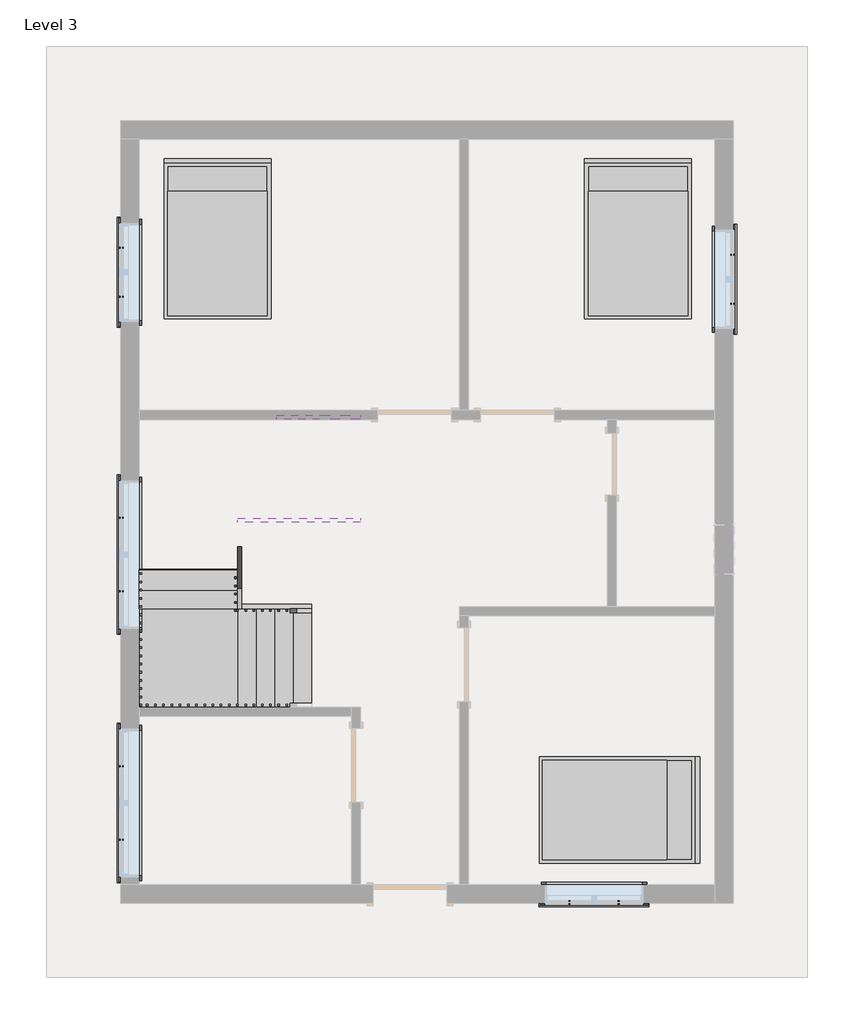
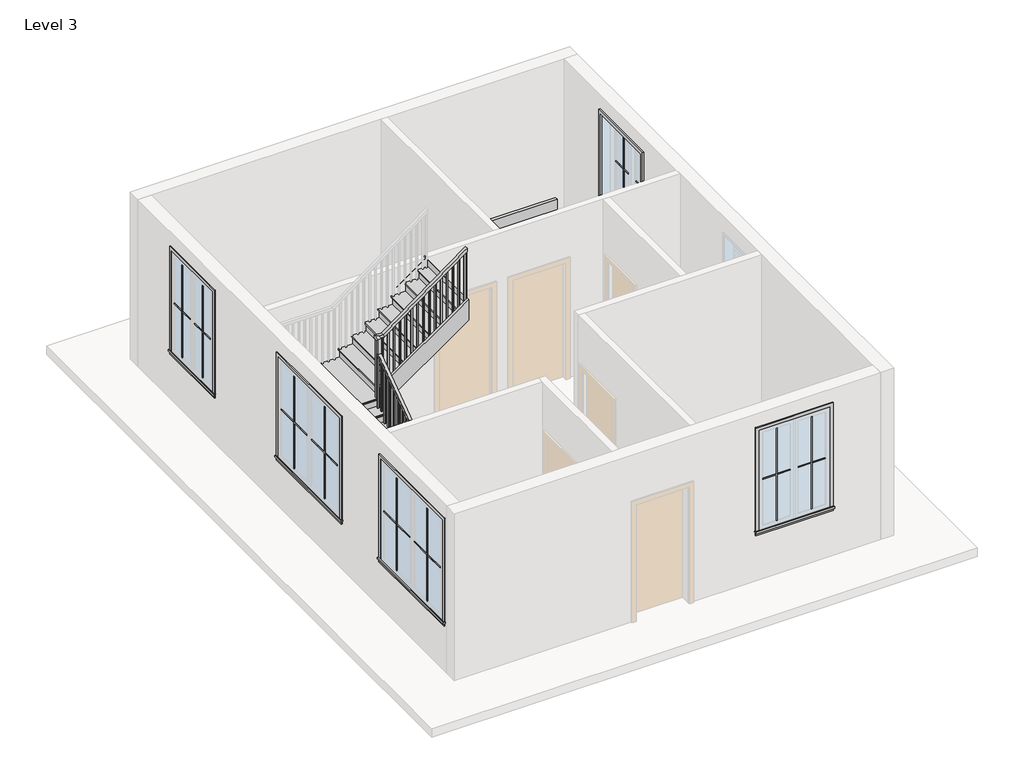
# One storey, part 3 of 3: 20 proxies, 5 members, 3 furniture elements, 1 railing, 1 stair flight.
"""IFC4 building model written with IfcOpenShell, lengths in millimetres."""

from ifc_helpers import new_model, si_unit, frame, origin, place, context, project, spatial, polyline, outline, extrude, faceted_brep, transform, mapped, element, save
from components import muntin_pattern_2x2_muntin_pattern_2x2_0a037076, muntin_pattern_2x2_muntin_pattern_2x2_e6f69628, muntin_pattern_2x2_muntin_pattern_2x2_2b4d9f72, muntin_pattern_2x2_muntin_pattern_2x2_ef995ed3, trim_window_exterior_flat_with_sill_b601e94a, trim_window_exterior_flat_with_sill_b7e4d11c, trim_window_interior_flat_picture_frame_bfefb25c, trim_window_interior_flat_picture_frame_936b8d2a, bed_17739_bed_17739_15c61121, stair_flight_424eac51

model = new_model("IFC4")

# Units and contexts
model_context = context("Model", 3, world=origin())
ifc_project = project(units=[si_unit("LENGTHUNIT", "METRE", prefix="MILLI")], contexts=[model_context])

# Site, building, storey
site = spatial("IfcSite", under=ifc_project)
building = spatial("IfcBuilding", under=site)
storey = spatial("IfcBuildingStorey", under=building, Name="Level 3", Elevation=6248.4)

# Proxies
placement = place(None, origin())
muntin_pattern_2x2_muntin_pattern_2x2_shape = muntin_pattern_2x2_muntin_pattern_2x2_0a037076(model_context)
element("IfcBuildingElementProxy", 1, Name="Muntin Pattern_2x2 : Muntin Pattern_2x2", ObjectType="Muntin Pattern_2x2 : Muntin Pattern_2x2", at=placement, inside=storey, context=model_context, shape_type="MappedRepresentation", body=[
    mapped(muntin_pattern_2x2_muntin_pattern_2x2_shape, transform((-5035.7855391, -4380.9248761, 7232.65), x_axis=(0.0, 1.0, 0.0), y_axis=(-1.0, 0.0, 0.0), z_axis=(0.0, 0.0, 1.0))),
])
element("IfcBuildingElementProxy", 2, Name="Muntin Pattern_2x2 : Muntin Pattern_2x2", ObjectType="Muntin Pattern_2x2 : Muntin Pattern_2x2", at=placement, inside=storey, context=model_context, shape_type="MappedRepresentation", body=[
    mapped(muntin_pattern_2x2_muntin_pattern_2x2_shape, transform((-5035.7855391, -1310.6998761, 7232.65), x_axis=(0.0, 1.0, 0.0), y_axis=(-1.0, 0.0, 0.0), z_axis=(0.0, 0.0, 1.0))),
])
muntin_pattern_2x2_muntin_pattern_2x2_2_shape = muntin_pattern_2x2_muntin_pattern_2x2_e6f69628(model_context)
element("IfcBuildingElementProxy", 3, Name="Muntin Pattern_2x2 : Muntin Pattern_2x2", ObjectType="Muntin Pattern_2x2 : Muntin Pattern_2x2", at=placement, inside=storey, context=model_context, shape_type="MappedRepresentation", body=[
    mapped(muntin_pattern_2x2_muntin_pattern_2x2_2_shape, transform((-5035.7855391, -3469.6998761, 7232.65), x_axis=(0.0, -1.0, 0.0), y_axis=(1.0, 0.0, 0.0), z_axis=(0.0, 0.0, 1.0))),
])
element("IfcBuildingElementProxy", 4, Name="Muntin Pattern_2x2 : Muntin Pattern_2x2", ObjectType="Muntin Pattern_2x2 : Muntin Pattern_2x2", at=placement, inside=storey, context=model_context, shape_type="MappedRepresentation", body=[
    mapped(muntin_pattern_2x2_muntin_pattern_2x2_2_shape, transform((-5035.7855391, -399.4748761, 7232.65), x_axis=(0.0, -1.0, 0.0), y_axis=(1.0, 0.0, 0.0), z_axis=(0.0, 0.0, 1.0))),
])
muntin_pattern_2x2_muntin_pattern_2x2_3_shape = muntin_pattern_2x2_muntin_pattern_2x2_2b4d9f72(model_context)
element("IfcBuildingElementProxy", 5, Name="Muntin Pattern_2x2 : Muntin Pattern_2x2", ObjectType="Muntin Pattern_2x2 : Muntin Pattern_2x2", at=placement, inside=storey, context=model_context, shape_type="MappedRepresentation", body=[
    mapped(muntin_pattern_2x2_muntin_pattern_2x2_3_shape, transform((1115.7769609, -5157.2123761, 7232.65), x_axis=(-1.0, 0.0, 0.0), y_axis=(0.0, -1.0, 0.0), z_axis=(0.0, 0.0, 1.0))),
])
element("IfcBuildingElementProxy", 6, Name="Muntin Pattern_2x2 : Muntin Pattern_2x2", ObjectType="Muntin Pattern_2x2 : Muntin Pattern_2x2", at=placement, inside=storey, context=model_context, shape_type="MappedRepresentation", body=[
    mapped(muntin_pattern_2x2_muntin_pattern_2x2_3_shape, transform((2527.0644609, 2851.7251239, 7232.65), x_axis=(0.0, -1.0, 0.0), y_axis=(1.0, 0.0, 0.0), z_axis=(0.0, 0.0, 1.0))),
])
element("IfcBuildingElementProxy", 7, Name="Muntin Pattern_2x2 : Muntin Pattern_2x2", ObjectType="Muntin Pattern_2x2 : Muntin Pattern_2x2", at=placement, inside=storey, context=model_context, shape_type="MappedRepresentation", body=[
    mapped(muntin_pattern_2x2_muntin_pattern_2x2_3_shape, transform((-5035.7855391, 2331.0251239, 7232.65), x_axis=(0.0, 1.0, 0.0), y_axis=(-1.0, 0.0, 0.0), z_axis=(0.0, 0.0, 1.0))),
])
muntin_pattern_2x2_muntin_pattern_2x2_4_shape = muntin_pattern_2x2_muntin_pattern_2x2_ef995ed3(model_context)
element("IfcBuildingElementProxy", 8, Name="Muntin Pattern_2x2 : Muntin Pattern_2x2", ObjectType="Muntin Pattern_2x2 : Muntin Pattern_2x2", at=placement, inside=storey, context=model_context, shape_type="MappedRepresentation", body=[
    mapped(muntin_pattern_2x2_muntin_pattern_2x2_4_shape, transform((509.3519609, -5157.2123761, 7232.65), x_axis=(1.0, 0.0, 0.0), y_axis=(0.0, 1.0, 0.0), z_axis=(0.0, 0.0, 1.0))),
])
element("IfcBuildingElementProxy", 9, Name="Muntin Pattern_2x2 : Muntin Pattern_2x2", ObjectType="Muntin Pattern_2x2 : Muntin Pattern_2x2", at=placement, inside=storey, context=model_context, shape_type="MappedRepresentation", body=[
    mapped(muntin_pattern_2x2_muntin_pattern_2x2_4_shape, transform((2527.0644609, 2245.3001239, 7232.65), x_axis=(0.0, 1.0, 0.0), y_axis=(-1.0, 0.0, 0.0), z_axis=(0.0, 0.0, 1.0))),
])
element("IfcBuildingElementProxy", 10, Name="Muntin Pattern_2x2 : Muntin Pattern_2x2", ObjectType="Muntin Pattern_2x2 : Muntin Pattern_2x2", at=placement, inside=storey, context=model_context, shape_type="MappedRepresentation", body=[
    mapped(muntin_pattern_2x2_muntin_pattern_2x2_4_shape, transform((-5035.7855391, 2937.4501239, 7232.65), x_axis=(0.0, -1.0, 0.0), y_axis=(1.0, 0.0, 0.0), z_axis=(0.0, 0.0, 1.0))),
])
trim_window_exterior_flat_with_sill_shape = trim_window_exterior_flat_with_sill_b601e94a(model_context)
element("IfcBuildingElementProxy", 11, Name="Trim-Window-Exterior-Flat : with Sill", ObjectType="Trim-Window-Exterior-Flat : with Sill", at=placement, inside=storey, context=model_context, shape_type="MappedRepresentation", body=[
    mapped(trim_window_exterior_flat_with_sill_shape, transform((-5045.3105391, -3925.3123761, 8991.6), x_axis=(0.0, -1.0, 0.0), y_axis=(0.0, 0.0, 1.0), z_axis=(-1.0, 0.0, 0.0))),
])
element("IfcBuildingElementProxy", 12, Name="Trim-Window-Exterior-Flat : with Sill", ObjectType="Trim-Window-Exterior-Flat : with Sill", at=placement, inside=storey, context=model_context, shape_type="MappedRepresentation", body=[
    mapped(trim_window_exterior_flat_with_sill_shape, transform((-5045.3105391, -855.0873761, 8991.6), x_axis=(0.0, -1.0, 0.0), y_axis=(0.0, 0.0, 1.0), z_axis=(-1.0, 0.0, 0.0))),
])
trim_window_exterior_flat_with_sill_2_shape = trim_window_exterior_flat_with_sill_b7e4d11c(model_context)
element("IfcBuildingElementProxy", 13, Name="Trim-Window-Exterior-Flat : with Sill", ObjectType="Trim-Window-Exterior-Flat : with Sill", at=placement, inside=storey, context=model_context, shape_type="MappedRepresentation", body=[
    mapped(trim_window_exterior_flat_with_sill_2_shape, transform((812.5644609, -5166.7373761, 8991.6), x_axis=(1.0, 0.0, 0.0), y_axis=(0.0, 0.0, 1.0), z_axis=(0.0, -1.0, 0.0))),
])
element("IfcBuildingElementProxy", 14, Name="Trim-Window-Exterior-Flat : with Sill", ObjectType="Trim-Window-Exterior-Flat : with Sill", at=placement, inside=storey, context=model_context, shape_type="MappedRepresentation", body=[
    mapped(trim_window_exterior_flat_with_sill_2_shape, transform((2536.5894609, 2548.5126239, 8991.6), x_axis=(0.0, 1.0, 0.0), y_axis=(0.0, 0.0, 1.0), z_axis=(1.0, 0.0, 0.0))),
])
element("IfcBuildingElementProxy", 15, Name="Trim-Window-Exterior-Flat : with Sill", ObjectType="Trim-Window-Exterior-Flat : with Sill", at=placement, inside=storey, context=model_context, shape_type="MappedRepresentation", body=[
    mapped(trim_window_exterior_flat_with_sill_2_shape, transform((-5045.3105391, 2634.2376239, 8991.6), x_axis=(0.0, -1.0, 0.0), y_axis=(0.0, 0.0, 1.0), z_axis=(-1.0, 0.0, 0.0))),
])
trim_window_interior_flat_picture_frame_shape = trim_window_interior_flat_picture_frame_bfefb25c(model_context)
element("IfcBuildingElementProxy", 16, Name="Trim-Window-Interior-Flat : Picture Frame", ObjectType="Trim-Window-Interior-Flat : Picture Frame", at=placement, inside=storey, context=model_context, shape_type="MappedRepresentation", body=[
    mapped(trim_window_interior_flat_picture_frame_shape, transform((-4816.7105391, -3925.3123761, 8991.6), x_axis=(0.0, 1.0, 0.0), y_axis=(0.0, 0.0, 1.0), z_axis=(1.0, 0.0, 0.0))),
])
element("IfcBuildingElementProxy", 17, Name="Trim-Window-Interior-Flat : Picture Frame", ObjectType="Trim-Window-Interior-Flat : Picture Frame", at=placement, inside=storey, context=model_context, shape_type="MappedRepresentation", body=[
    mapped(trim_window_interior_flat_picture_frame_shape, transform((-4816.7105391, -855.0873761, 8991.6), x_axis=(0.0, 1.0, 0.0), y_axis=(0.0, 0.0, 1.0), z_axis=(1.0, 0.0, 0.0))),
])
trim_window_interior_flat_picture_frame_2_shape = trim_window_interior_flat_picture_frame_936b8d2a(model_context)
element("IfcBuildingElementProxy", 18, Name="Trim-Window-Interior-Flat : Picture Frame", ObjectType="Trim-Window-Interior-Flat : Picture Frame", at=placement, inside=storey, context=model_context, shape_type="MappedRepresentation", body=[
    mapped(trim_window_interior_flat_picture_frame_2_shape, transform((812.5644609, -4938.1373761, 8991.6), x_axis=(-1.0, 0.0, 0.0), y_axis=(0.0, 0.0, 1.0), z_axis=(0.0, 1.0, 0.0))),
])
element("IfcBuildingElementProxy", 19, Name="Trim-Window-Interior-Flat : Picture Frame", ObjectType="Trim-Window-Interior-Flat : Picture Frame", at=placement, inside=storey, context=model_context, shape_type="MappedRepresentation", body=[
    mapped(trim_window_interior_flat_picture_frame_2_shape, transform((2307.9894609, 2548.5126239, 8991.6), x_axis=(0.0, -1.0, 0.0), y_axis=(0.0, 0.0, 1.0), z_axis=(-1.0, 0.0, 0.0))),
])
element("IfcBuildingElementProxy", 20, Name="Trim-Window-Interior-Flat : Picture Frame", ObjectType="Trim-Window-Interior-Flat : Picture Frame", at=placement, inside=storey, context=model_context, shape_type="MappedRepresentation", body=[
    mapped(trim_window_interior_flat_picture_frame_2_shape, transform((-4816.7105391, 2634.2376239, 8991.6), x_axis=(0.0, 1.0, 0.0), y_axis=(0.0, 0.0, 1.0), z_axis=(1.0, 0.0, 0.0))),
])

# Furniture
bed_17739_bed_17739_shape = bed_17739_bed_17739_15c61121(model_context)
element("IfcFurniture", 21, ObjectType="Bed_17739 : Bed_17739", at=placement, inside=storey, context=model_context, shape_type="MappedRepresentation", body=[
    mapped(bed_17739_bed_17739_shape, transform((-3845.1605391, 3024.7626239, 6248.4), x_axis=(1.0, 0.0, 0.0), y_axis=(0.0, 1.0, 0.0), z_axis=(0.0, 0.0, 1.0))),
])
element("IfcFurniture", 22, ObjectType="Bed_17739 : Bed_17739", at=placement, inside=storey, context=model_context, shape_type="MappedRepresentation", body=[
    mapped(bed_17739_bed_17739_shape, transform((1355.4894609, 3024.7626239, 6248.4), x_axis=(1.0, 0.0, 0.0), y_axis=(0.0, 1.0, 0.0), z_axis=(0.0, 0.0, 1.0))),
])
element("IfcFurniture", 23, ObjectType="Bed_17739 : Bed_17739", at=placement, inside=storey, context=model_context, shape_type="MappedRepresentation", body=[
    mapped(bed_17739_bed_17739_shape, transform((1101.4894609, -4011.0373761, 6248.4), x_axis=(0.0, -1.0, 0.0), y_axis=(1.0, 0.0, 0.0), z_axis=(0.0, 0.0, 1.0))),
])

# Members
element("IfcMember", 24, ObjectType="Stringer - 2\" Width", at=placement, inside=storey, context=model_context, shape_type="SweptSolid", body=[
    extrude(outline(polyline([(6248.4, -2683.1105391), (6398.9087903, -2683.1105391), (6398.9087903, -3112.2707489), (6248.4, -2897.7957228), (6248.4, -2683.1105391)])), frame((0.0, -2791.8373761, 0.0), z_axis=(0.0, 1.0, 0.0), x_axis=(0.0, 0.0, 1.0)), (0.0, 0.0, 1.0), 50.8),
])
element("IfcMember", 25, ObjectType="Stringer - 2\" Width", at=placement, inside=storey, context=model_context, shape_type="SweptSolid", body=[
    extrude(outline(polyline([(8575.8856495, -2580.7583047), (8931.8489938, -2073.5105391), (9304.2117181, -2073.5105391), (8575.8856495, -3111.3751869), (8575.8856495, -2580.7583047)])), frame((0.0, 814.9626239, 0.0), z_axis=(0.0, 1.0, 0.0), x_axis=(0.0, 0.0, 1.0)), (0.0, 0.0, 1.0), 50.8),
])
element("IfcMember", 26, ObjectType="Stringer - 2\" Width", at=placement, inside=storey, context=model_context, shape_type="SweptSolid", body=[
    extrude(outline(polyline([(6248.4, -2683.1105391), (6470.106455, -2683.1105391), (7076.1415427, -3546.7105391), (6703.7788184, -3546.7105391), (6248.4, -2897.7957228), (6248.4, -2683.1105391)])), frame((0.0, -1521.8373761, 0.0), z_axis=(0.0, 1.0, 0.0), x_axis=(0.0, 0.0, 1.0)), (0.0, 0.0, 1.0), 50.8),
])
element("IfcMember", 27, ObjectType="Stringer - 2\" Width", at=placement, inside=storey, context=model_context, shape_type="SweptSolid", body=[
    extrude(outline(polyline([(-1521.8373761, 6898.7564629), (-1521.8373761, 7273.9327137), (-455.0373761, 8039.5786467), (-455.0373761, 7664.4023959), (-1521.8373761, 6898.7564629)])), frame((-3597.5105391, 0.0, 0.0), z_axis=(1.0, 0.0, 0.0), x_axis=(0.0, 1.0, 0.0)), (0.0, 0.0, 1.0), 50.8),
])
element("IfcMember", 28, ObjectType="Stringer - 2\" Width", at=placement, inside=storey, context=model_context, shape_type="SweptSolid", body=[
    extrude(outline(polyline([(8234.7380339, -3597.5105391), (7862.3753096, -3597.5105391), (8931.8489938, -2073.5105391), (9304.2117181, -2073.5105391), (8234.7380339, -3597.5105391)])), frame((0.0, -455.0373761, 0.0), z_axis=(0.0, 1.0, 0.0), x_axis=(0.0, 0.0, 1.0)), (0.0, 0.0, 1.0), 50.8),
])

# Railing
element("IfcRailing", 29, ObjectType="Handrail - Rectangular", at=placement, inside=storey, context=model_context, shape_type="SolidModel", body=[
    faceted_brep([(-2683.1105391, -1572.6373761, 7323.2210526), (-2683.1105391, -1572.6373761, 7261.1605986), (-2683.1105391, -1521.8373761, 7261.1605986), (-2683.1105391, -1521.8373761, 7323.2210526), (-3521.3105391, -1572.6373761, 7911.4315789), (-3572.1105391, -1572.6373761, 7885.0202477), (-3572.1105391, -1521.8373761, 7885.0202477), (-3521.3105391, -1521.8373761, 7911.4315789), (-3521.3105391, -1572.6373761, 8180.015311), (-3572.1105391, -1572.6373761, 8129.215311), (-3572.1105391, -1521.8373761, 8129.215311), (-3521.3105391, -1521.8373761, 8180.015311), (-3648.3105391, -1572.6373761, 8180.015311), (-3648.3105391, -1572.6373761, 8129.215311), (-3597.5105391, -1521.8373761, 8129.215311), (-3597.5105391, -1521.8373761, 8180.015311), (-3648.3105391, -1445.6373761, 8180.015311), (-3648.3105391, -1429.2944467, 8129.215311), (-3597.5105391, -1429.2944467, 8129.215311), (-3597.5105391, -1445.6373761, 8180.015311), (-3648.3105391, -480.4373761, 8872.7425837), (-3648.3105391, -429.6373761, 8846.6725387), (-3597.5105391, -429.6373761, 8846.6725387), (-3597.5105391, -480.4373761, 8872.7425837), (-3648.3105391, -480.4373761, 9144.0), (-3648.3105391, -429.6373761, 9093.2), (-3597.5105391, -429.6373761, 9093.2), (-3597.5105391, -480.4373761, 9144.0), (-3648.3105391, -353.4373761, 9144.0), (-3648.3105391, -353.4373761, 9093.2), (-3597.5105391, -404.2373761, 9093.2), (-3597.5105391, -404.2373761, 9144.0), (-3521.3105391, -353.4373761, 9144.0), (-3504.6160355, -353.4373761, 9093.2), (-3504.6160355, -404.2373761, 9093.2), (-3521.3105391, -404.2373761, 9144.0), (-2073.5105391, -353.4373761, 10210.8), (-2073.5105391, -404.2373761, 10210.8), (-2073.5105391, -404.2373761, 10147.6987868), (-2073.5105391, -353.4373761, 10147.6987868)], [[[0, 1, 2, 3]], [[1, 0, 4, 5]], [[2, 1, 5, 6]], [[3, 2, 6, 7]], [[0, 3, 7, 4]], [[5, 4, 8, 9]], [[6, 5, 9, 10]], [[7, 6, 10, 11]], [[4, 7, 11, 8]], [[9, 8, 12, 13]], [[10, 9, 13, 14]], [[11, 10, 14, 15]], [[8, 11, 15, 12]], [[13, 12, 16, 17]], [[14, 13, 17, 18]], [[15, 14, 18, 19]], [[12, 15, 19, 16]], [[17, 16, 20, 21]], [[18, 17, 21, 22]], [[19, 18, 22, 23]], [[16, 19, 23, 20]], [[21, 20, 24, 25]], [[22, 21, 25, 26]], [[23, 22, 26, 27]], [[20, 23, 27, 24]], [[25, 24, 28, 29]], [[26, 25, 29, 30]], [[27, 26, 30, 31]], [[24, 27, 31, 28]], [[29, 28, 32, 33]], [[30, 29, 33, 34]], [[31, 30, 34, 35]], [[28, 31, 35, 32]], [[36, 37, 38, 39]], [[33, 32, 36, 39]], [[34, 33, 39, 38]], [[35, 34, 38, 37]], [[32, 35, 37, 36]]]),
    extrude(outline(polyline([(10136.0014184, -2089.3855391), (10121.9645763, -2108.4355391), (9135.9789474, -2108.4355391), (9135.9789474, -2089.3855391), (10136.0014184, -2089.3855391)])), frame((0.0, -388.3623761, 0.0), z_axis=(0.0, 1.0, 0.0), x_axis=(0.0, 0.0, 1.0)), (0.0, 0.0, 1.0), 19.05),
    extrude(outline(polyline([(10061.1382605, -2190.9855391), (10047.1014184, -2210.0355391), (9135.9789474, -2210.0355391), (9135.9789474, -2190.9855391), (10061.1382605, -2190.9855391)])), frame((0.0, -388.3623761, 0.0), z_axis=(0.0, 1.0, 0.0), x_axis=(0.0, 0.0, 1.0)), (0.0, 0.0, 1.0), 19.05),
    extrude(outline(polyline([(9986.2751026, -2292.5855391), (9972.2382605, -2311.6355391), (8975.5578947, -2311.6355391), (8975.5578947, -2292.5855391), (9986.2751026, -2292.5855391)])), frame((0.0, -388.3623761, 0.0), z_axis=(0.0, 1.0, 0.0), x_axis=(0.0, 0.0, 1.0)), (0.0, 0.0, 1.0), 19.05),
    extrude(outline(polyline([(9911.4119447, -2394.1855391), (9897.3751026, -2413.2355391), (8975.5578947, -2413.2355391), (8975.5578947, -2394.1855391), (9911.4119447, -2394.1855391)])), frame((0.0, -388.3623761, 0.0), z_axis=(0.0, 1.0, 0.0), x_axis=(0.0, 0.0, 1.0)), (0.0, 0.0, 1.0), 19.05),
    extrude(outline(polyline([(9836.5487868, -2495.7855391), (9822.5119447, -2514.8355391), (8815.1368421, -2514.8355391), (8815.1368421, -2495.7855391), (9836.5487868, -2495.7855391)])), frame((0.0, -388.3623761, 0.0), z_axis=(0.0, 1.0, 0.0), x_axis=(0.0, 0.0, 1.0)), (0.0, 0.0, 1.0), 19.05),
    extrude(outline(polyline([(9761.6856289, -2597.3855391), (9747.6487868, -2616.4355391), (8815.1368421, -2616.4355391), (8815.1368421, -2597.3855391), (9761.6856289, -2597.3855391)])), frame((0.0, -388.3623761, 0.0), z_axis=(0.0, 1.0, 0.0), x_axis=(0.0, 0.0, 1.0)), (0.0, 0.0, 1.0), 19.05),
    extrude(outline(polyline([(9686.822471, -2698.9855391), (9672.7856289, -2718.0355391), (8654.7157895, -2718.0355391), (8654.7157895, -2698.9855391), (9686.822471, -2698.9855391)])), frame((0.0, -388.3623761, 0.0), z_axis=(0.0, 1.0, 0.0), x_axis=(0.0, 0.0, 1.0)), (0.0, 0.0, 1.0), 19.05),
    extrude(outline(polyline([(9611.9593132, -2800.5855391), (9597.922471, -2819.6355391), (8654.7157895, -2819.6355391), (8654.7157895, -2800.5855391), (9611.9593132, -2800.5855391)])), frame((0.0, -388.3623761, 0.0), z_axis=(0.0, 1.0, 0.0), x_axis=(0.0, 0.0, 1.0)), (0.0, 0.0, 1.0), 19.05),
    extrude(outline(polyline([(9537.0961553, -2902.1855391), (9523.0593132, -2921.2355391), (8654.7157895, -2921.2355391), (8654.7157895, -2902.1855391), (9537.0961553, -2902.1855391)])), frame((0.0, -388.3623761, 0.0), z_axis=(0.0, 1.0, 0.0), x_axis=(0.0, 0.0, 1.0)), (0.0, 0.0, 1.0), 19.05),
    extrude(outline(polyline([(9462.2329974, -3003.7855391), (9448.1961553, -3022.8355391), (8494.2947368, -3022.8355391), (8494.2947368, -3003.7855391), (9462.2329974, -3003.7855391)])), frame((0.0, -388.3623761, 0.0), z_axis=(0.0, 1.0, 0.0), x_axis=(0.0, 0.0, 1.0)), (0.0, 0.0, 1.0), 19.05),
    extrude(outline(polyline([(9387.3698395, -3105.3855391), (9373.3329974, -3124.4355391), (8494.2947368, -3124.4355391), (8494.2947368, -3105.3855391), (9387.3698395, -3105.3855391)])), frame((0.0, -388.3623761, 0.0), z_axis=(0.0, 1.0, 0.0), x_axis=(0.0, 0.0, 1.0)), (0.0, 0.0, 1.0), 19.05),
    extrude(outline(polyline([(9312.5066816, -3206.9855391), (9298.4698395, -3226.0355391), (8333.8736842, -3226.0355391), (8333.8736842, -3206.9855391), (9312.5066816, -3206.9855391)])), frame((0.0, -388.3623761, 0.0), z_axis=(0.0, 1.0, 0.0), x_axis=(0.0, 0.0, 1.0)), (0.0, 0.0, 1.0), 19.05),
    extrude(outline(polyline([(9237.6435237, -3308.5855391), (9223.6066816, -3327.6355391), (8333.8736842, -3327.6355391), (8333.8736842, -3308.5855391), (9237.6435237, -3308.5855391)])), frame((0.0, -388.3623761, 0.0), z_axis=(0.0, 1.0, 0.0), x_axis=(0.0, 0.0, 1.0)), (0.0, 0.0, 1.0), 19.05),
    extrude(outline(polyline([(9162.7803658, -3410.1855391), (9148.7435237, -3429.2355391), (8173.4526316, -3429.2355391), (8173.4526316, -3410.1855391), (9162.7803658, -3410.1855391)])), frame((0.0, -388.3623761, 0.0), z_axis=(0.0, 1.0, 0.0), x_axis=(0.0, 0.0, 1.0)), (0.0, 0.0, 1.0), 19.05),
    extrude(outline(polyline([(9087.9172079, -3511.7855391), (9073.8803658, -3530.8355391), (8173.4526316, -3530.8355391), (8173.4526316, -3511.7855391), (9087.9172079, -3511.7855391)])), frame((0.0, -388.3623761, 0.0), z_axis=(0.0, 1.0, 0.0), x_axis=(0.0, 0.0, 1.0)), (0.0, 0.0, 1.0), 19.05),
    extrude(outline(polyline([(-3613.3855391, -439.1623761), (-3632.4355391, -439.1623761), (-3632.4355391, -420.1123761), (-3613.3855391, -420.1123761), (-3613.3855391, -439.1623761)])), frame((0.0, 0.0, 7852.6105263), z_axis=(0.0, 0.0, 1.0), x_axis=(1.0, 0.0, 0.0)), (0.0, 0.0, 1.0), 1240.5894737),
    extrude(outline(polyline([(-540.7623761, 8766.9177541), (-521.7123761, 8780.5900029), (-521.7123761, 7852.6105263), (-540.7623761, 7852.6105263), (-540.7623761, 8766.9177541)])), frame((-3632.4355391, 0.0, 0.0), z_axis=(1.0, 0.0, 0.0), x_axis=(0.0, 1.0, 0.0)), (0.0, 0.0, 1.0), 19.05),
    extrude(outline(polyline([(-642.3623761, 8693.9990938), (-623.3123761, 8707.6713426), (-623.3123761, 7692.1894737), (-642.3623761, 7692.1894737), (-642.3623761, 8693.9990938)])), frame((-3632.4355391, 0.0, 0.0), z_axis=(1.0, 0.0, 0.0), x_axis=(0.0, 1.0, 0.0)), (0.0, 0.0, 1.0), 19.05),
    extrude(outline(polyline([(-743.9623761, 8621.0804335), (-724.9123761, 8634.7526823), (-724.9123761, 7692.1894737), (-743.9623761, 7692.1894737), (-743.9623761, 8621.0804335)])), frame((-3632.4355391, 0.0, 0.0), z_axis=(1.0, 0.0, 0.0), x_axis=(0.0, 1.0, 0.0)), (0.0, 0.0, 1.0), 19.05),
    extrude(outline(polyline([(-845.5623761, 8548.1617732), (-826.5123761, 8561.834022), (-826.5123761, 7692.1894737), (-845.5623761, 7692.1894737), (-845.5623761, 8548.1617732)])), frame((-3632.4355391, 0.0, 0.0), z_axis=(1.0, 0.0, 0.0), x_axis=(0.0, 1.0, 0.0)), (0.0, 0.0, 1.0), 19.05),
    extrude(outline(polyline([(-947.1623761, 8475.2431129), (-928.1123761, 8488.9153617), (-928.1123761, 7531.7684211), (-947.1623761, 7531.7684211), (-947.1623761, 8475.2431129)])), frame((-3632.4355391, 0.0, 0.0), z_axis=(1.0, 0.0, 0.0), x_axis=(0.0, 1.0, 0.0)), (0.0, 0.0, 1.0), 19.05),
    extrude(outline(polyline([(-1048.7623761, 8402.3244526), (-1029.7123761, 8415.9967014), (-1029.7123761, 7531.7684211), (-1048.7623761, 7531.7684211), (-1048.7623761, 8402.3244526)])), frame((-3632.4355391, 0.0, 0.0), z_axis=(1.0, 0.0, 0.0), x_axis=(0.0, 1.0, 0.0)), (0.0, 0.0, 1.0), 19.05),
    extrude(outline(polyline([(-1150.3623761, 8329.4057923), (-1131.3123761, 8343.0780411), (-1131.3123761, 7371.3473684), (-1150.3623761, 7371.3473684), (-1150.3623761, 8329.4057923)])), frame((-3632.4355391, 0.0, 0.0), z_axis=(1.0, 0.0, 0.0), x_axis=(0.0, 1.0, 0.0)), (0.0, 0.0, 1.0), 19.05),
    extrude(outline(polyline([(-1251.9623761, 8256.487132), (-1232.9123761, 8270.1593808), (-1232.9123761, 7371.3473684), (-1251.9623761, 7371.3473684), (-1251.9623761, 8256.487132)])), frame((-3632.4355391, 0.0, 0.0), z_axis=(1.0, 0.0, 0.0), x_axis=(0.0, 1.0, 0.0)), (0.0, 0.0, 1.0), 19.05),
    extrude(outline(polyline([(-1353.5623761, 8183.5684718), (-1334.5123761, 8197.2407206), (-1334.5123761, 7210.9263158), (-1353.5623761, 7210.9263158), (-1353.5623761, 8183.5684718)])), frame((-3632.4355391, 0.0, 0.0), z_axis=(1.0, 0.0, 0.0), x_axis=(0.0, 1.0, 0.0)), (0.0, 0.0, 1.0), 19.05),
    extrude(outline(polyline([(-1455.1623761, 8110.6498115), (-1436.1123761, 8124.3220603), (-1436.1123761, 7210.9263158), (-1455.1623761, 7210.9263158), (-1455.1623761, 8110.6498115)])), frame((-3632.4355391, 0.0, 0.0), z_axis=(1.0, 0.0, 0.0), x_axis=(0.0, 1.0, 0.0)), (0.0, 0.0, 1.0), 19.05),
    extrude(outline(polyline([(-3587.9855391, -1537.7123761), (-3587.9855391, -1556.7623761), (-3607.0355391, -1556.7623761), (-3607.0355391, -1537.7123761), (-3587.9855391, -1537.7123761)])), frame((0.0, 0.0, 7050.5052632), z_axis=(0.0, 0.0, 1.0), x_axis=(1.0, 0.0, 0.0)), (0.0, 0.0, 1.0), 1078.7100478),
    extrude(outline(polyline([(7824.862353, -3486.3855391), (7838.230774, -3505.4355391), (6890.0842105, -3505.4355391), (6890.0842105, -3486.3855391), (7824.862353, -3486.3855391)])), frame((0.0, -1556.7623761, 0.0), z_axis=(0.0, 1.0, 0.0), x_axis=(0.0, 0.0, 1.0)), (0.0, 0.0, 1.0), 19.05),
    extrude(outline(polyline([(7753.5641074, -3384.7855391), (7766.9325284, -3403.8355391), (6890.0842105, -3403.8355391), (6890.0842105, -3384.7855391), (7753.5641074, -3384.7855391)])), frame((0.0, -1556.7623761, 0.0), z_axis=(0.0, 1.0, 0.0), x_axis=(0.0, 0.0, 1.0)), (0.0, 0.0, 1.0), 19.05),
    extrude(outline(polyline([(7682.2658617, -3283.1855391), (7695.6342828, -3302.2355391), (6729.6631579, -3302.2355391), (6729.6631579, -3283.1855391), (7682.2658617, -3283.1855391)])), frame((0.0, -1556.7623761, 0.0), z_axis=(0.0, 1.0, 0.0), x_axis=(0.0, 0.0, 1.0)), (0.0, 0.0, 1.0), 19.05),
    extrude(outline(polyline([(7610.9676161, -3181.5855391), (7624.3360372, -3200.6355391), (6729.6631579, -3200.6355391), (6729.6631579, -3181.5855391), (7610.9676161, -3181.5855391)])), frame((0.0, -1556.7623761, 0.0), z_axis=(0.0, 1.0, 0.0), x_axis=(0.0, 0.0, 1.0)), (0.0, 0.0, 1.0), 19.05),
    extrude(outline(polyline([(7539.6693705, -3079.9855391), (7553.0377916, -3099.0355391), (6569.2421053, -3099.0355391), (6569.2421053, -3079.9855391), (7539.6693705, -3079.9855391)])), frame((0.0, -1556.7623761, 0.0), z_axis=(0.0, 1.0, 0.0), x_axis=(0.0, 0.0, 1.0)), (0.0, 0.0, 1.0), 19.05),
    extrude(outline(polyline([(7468.3711249, -2978.3855391), (7481.7395459, -2997.4355391), (6569.2421053, -2997.4355391), (6569.2421053, -2978.3855391), (7468.3711249, -2978.3855391)])), frame((0.0, -1556.7623761, 0.0), z_axis=(0.0, 1.0, 0.0), x_axis=(0.0, 0.0, 1.0)), (0.0, 0.0, 1.0), 19.05),
    extrude(outline(polyline([(7397.0728793, -2876.7855391), (7410.4413003, -2895.8355391), (6408.8210526, -2895.8355391), (6408.8210526, -2876.7855391), (7397.0728793, -2876.7855391)])), frame((0.0, -1556.7623761, 0.0), z_axis=(0.0, 1.0, 0.0), x_axis=(0.0, 0.0, 1.0)), (0.0, 0.0, 1.0), 19.05),
    extrude(outline(polyline([(7325.7746337, -2775.1855391), (7339.1430547, -2794.2355391), (6408.8210526, -2794.2355391), (6408.8210526, -2775.1855391), (7325.7746337, -2775.1855391)])), frame((0.0, -1556.7623761, 0.0), z_axis=(0.0, 1.0, 0.0), x_axis=(0.0, 0.0, 1.0)), (0.0, 0.0, 1.0), 19.05),
    extrude(outline(polyline([(-3613.3855391, -388.3623761), (-3632.4355391, -388.3623761), (-3632.4355391, -369.3123761), (-3613.3855391, -369.3123761), (-3613.3855391, -388.3623761)])), frame((0.0, 0.0, 8013.0315789), z_axis=(0.0, 0.0, 1.0), x_axis=(1.0, 0.0, 0.0)), (0.0, 0.0, 1.0), 1080.1684211),
    extrude(outline(polyline([(-3613.3855391, -1537.7123761), (-3613.3855391, -1556.7623761), (-3632.4355391, -1556.7623761), (-3632.4355391, -1537.7123761), (-3613.3855391, -1537.7123761)])), frame((0.0, 0.0, 7050.5052632), z_axis=(0.0, 0.0, 1.0), x_axis=(1.0, 0.0, 0.0)), (0.0, 0.0, 1.0), 1078.7100478),
    extrude(outline(polyline([(10147.6987868, -2073.5105391), (10133.6619447, -2092.5605391), (9135.9789474, -2092.5605391), (9135.9789474, -2073.5105391), (10147.6987868, -2073.5105391)])), frame((0.0, -388.3623761, 0.0), z_axis=(0.0, 1.0, 0.0), x_axis=(0.0, 0.0, 1.0)), (0.0, 0.0, 1.0), 19.05),
    extrude(outline(polyline([(7261.1605986, -2683.1105391), (7274.5290196, -2702.1605391), (6408.8210526, -2702.1605391), (6408.8210526, -2683.1105391), (7261.1605986, -2683.1105391)])), frame((0.0, -1556.7623761, 0.0), z_axis=(0.0, 1.0, 0.0), x_axis=(0.0, 0.0, 1.0)), (0.0, 0.0, 1.0), 19.05),
])

# Stair flight
stair_flight_shape = stair_flight_424eac51(model_context)
element("IfcStairFlight", 30, ObjectType="2\" Tread 1\" Nosing 1/4\" Riser", at=placement, inside=storey, context=model_context, shape_type="MappedRepresentation", body=[
    mapped(stair_flight_shape, transform((0.0, 0.0, 0.0), x_axis=(1.0, 0.0, 0.0), y_axis=(0.0, 1.0, 0.0), z_axis=(0.0, 0.0, 1.0))),
])

save(model, "model.ifc")

# Revit data of these elements
# Type "Muntin Pattern_2x2 : Muntin Pattern_2x2"
#   Width [instance default] = 4' - 0"
#   Thickness = 0' - 0 1/2"
#   Height [instance default] = 4' - 0"
#   Distance = 0' - 0 3/4"
#   Interior Material [instance default] = none
#   Exterior Material [instance default] = none
#   Default Elevation = 0
# Type "Trim-Window-Exterior-Flat : with Sill"
#   Trim Width = 0' - 2 1/4"
#   Trim Thickness_Picture Frame = 0' - 1 1/4"
#   Trim Thickness_with Sill = 0' - 0 3/4"
#   Sill Thickness = 0' - 1 1/4"
#   Opening Width [instance default] = 2' - 0"
#   Opening Height [instance default] = 3' - 0"
#   Default Elevation = 4' - 0"
#   Sill = yes
#   Picture Frame = no
#   Trim Material [instance default] = none
# Type "Trim-Window-Interior-Flat : Picture Frame"
#   Trim Thickness_Picture Frame = 0' - 1 1/4"
#   Trim Width = 0' - 2 1/4"
#   Trim Thickness_with Sill = 0' - 0 3/4"
#   Sill Thickness = 0' - 1 1/4"
#   Opening Width [instance default] = 2' - 0"
#   Opening Height [instance default] = 3' - 0"
#   Default Elevation = 4' - 0"
#   Sill = no
#   Picture Frame = yes
#   Trim Material [instance default] = none
# Type "Bed_17739 : Bed_17739"
#   Default Elevation = 0
# Type "Handrail - Rectangular"
#   Assembly Code = "C2010400"
#   built-in parameter 1008612 = 0.0416667 (stored number, unit not read)
#   built-in parameter 1008611 = 0.0416667 (stored number, unit not read)
#   built-in parameter 1008609 = 0.333333 (stored number, unit not read)
#   built-in parameter 1008604 = 0.166667 (stored number, unit not read)
#   built-in parameter 1008603 = 0.166667 (stored number, unit not read)
#   Railing Height = 3' - 0"
#   built-in parameter 1008630 = 2
#   built-in parameter 1008610 = 2
#   built-in parameter 1008618 = Baluster - Square : 3/4"
# Elements 1, 2, 3, 4 (IfcBuildingElementProxy, "Muntin Pattern_2x2 : Muntin Pattern_2x2")
#   Width = 2' - 6 5/8"
#   Height = 5' - 6 1/2"
#   Interior Material = Wood - Stained
#   Exterior Material = Clad - White
#   Phase Created = New Construction
#   Materials on its faces: "Clad - White", "Wood - Stained"
# Elements 5, 6, 7, 8, 9, 10 (IfcBuildingElementProxy, "Muntin Pattern_2x2 : Muntin Pattern_2x2")
#   Width = 1' - 6 5/8"
#   Height = 5' - 6 1/2"
#   Interior Material = Wood - Stained
#   Exterior Material = Clad - White
#   Phase Created = New Construction
#   Materials on its faces: "Clad - White", "Wood - Stained"
# Elements 11, 12 (IfcBuildingElementProxy, "Trim-Window-Exterior-Flat : with Sill")
#   Opening Width = 6' - 0"
#   Opening Height = 6' - 0"
#   Trim Material = Clad - White
#   Phase Created = New Construction
#   Materials on its faces: "Clad - White"
# Elements 13, 14, 15 (IfcBuildingElementProxy, "Trim-Window-Exterior-Flat : with Sill")
#   Opening Width = 4' - 0"
#   Opening Height = 6' - 0"
#   Trim Material = Clad - White
#   Phase Created = New Construction
#   Materials on its faces: "Clad - White"
# Elements 16, 17 (IfcBuildingElementProxy, "Trim-Window-Interior-Flat : Picture Frame")
#   Opening Width = 6' - 0"
#   Opening Height = 6' - 0"
#   Trim Material = Wood - Stained
#   Phase Created = New Construction
#   Materials on its faces: "Wood - Stained"
# Elements 18, 19, 20 (IfcBuildingElementProxy, "Trim-Window-Interior-Flat : Picture Frame")
#   Opening Width = 4' - 0"
#   Opening Height = 6' - 0"
#   Trim Material = Wood - Stained
#   Phase Created = New Construction
#   Materials on its faces: "Wood - Stained"
# Elements 21, 22, 23 (IfcFurniture, "Bed_17739 : Bed_17739")
#   Phase Created = New Construction
#   Materials on its faces: "legs", "sheets", "bed frame", "Blanket"
# Elements 24, 25, 26, 27, 28 (IfcMember, "Stringer - 2\" Width")
#   Phase Created = New Construction
# Element 29 (IfcRailing, "Handrail - Rectangular")
#   Phase Created = New Construction
# Element 30 (IfcStairFlight, "2\" Tread 1\" Nosing 1/4\" Riser")
#   Phase Created = New Construction
# Materials
#   "Clad - White": class "Wood", colour RGB 242 242 238, transparency 0, Cost = 0
#   "Wood - Stained": class "Wood", colour RGB 224 178 126, transparency 0, Cost = 0
#   "legs": colour RGB 90 73 37, transparency 0, Cost = 0
#   "sheets": colour RGB 200 195 176, transparency 0, Cost = 0
#   "bed frame": colour RGB 90 73 37, transparency 0, Cost = 0
#   "Blanket": class "System", colour RGB 59 0 1, transparency 0, Cost = 0
